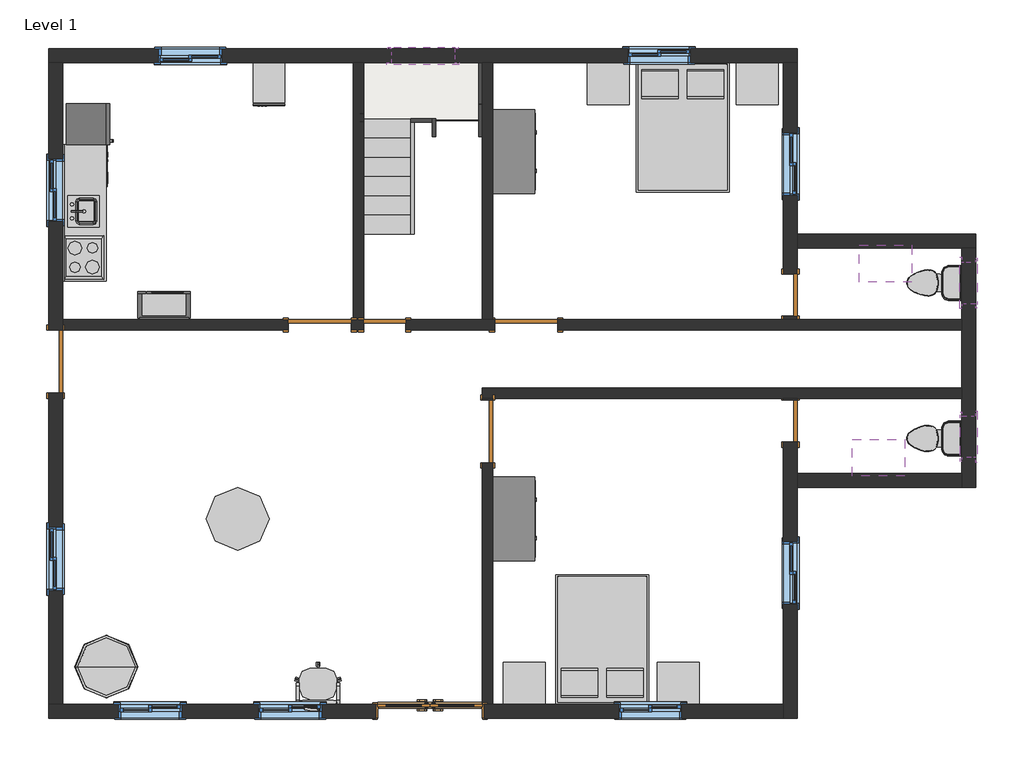
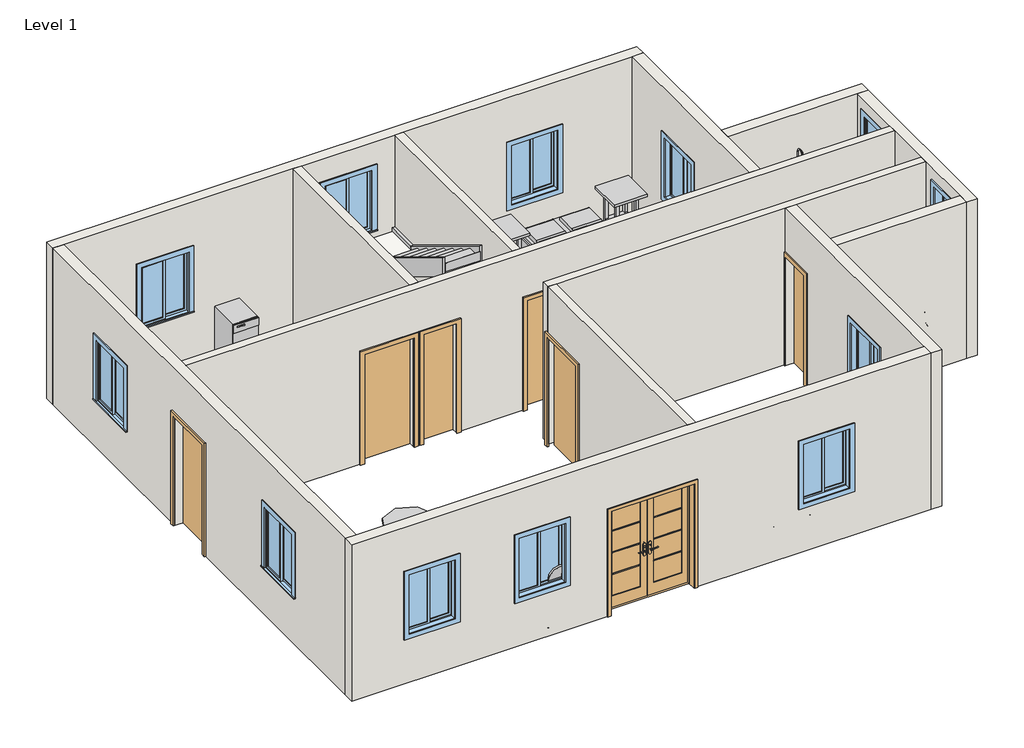
# One storey, incomplete: 13 walls, 12 furniture elements, 12 windows, 8 doors, 8 members, 6 proxies, 5 flow terminals, 2 stair flights, 1 slab.
"""IFC4 building model written with IfcOpenShell, lengths in millimetres."""

from ifc_helpers import new_model, si_unit, frame, origin, origin_with_axes, place, context, project, spatial, polyline, outline, extrude, faceted_brep, transform, mapped, element, save
from components import proxy_7e1014cc, proxy_a6faaae8, proxy_45b28599, kitchenette_medium_kitchenette_medium_844211aa, proxy_8a8d5ab2, proxy_c523a7b7, door_b03bd389, door_16372e1c, door_686f89d2, door_719f80de, single_flush_inner_door_2_1112daf7, single_flush_inner_door_2_89112ad5, single_flush_inner_door_2_5ca4d175, flow_terminal_871c2e40, flow_terminal_38af2918, toilet_domestic_3d_toilet_domestic_3d_f7549cf7, toilet_domestic_3d_toilet_domestic_3d_183bbd19, furniture_c8abb964, chair_executive_chair_executive_8d69e98c, furniture_c6510c7c, furniture_9fa109b2, furniture_905aceb5, furniture_5bc9ed15, furniture_c80d6d9c, non_monolithic_landing_d6ac0f27, stair_flight_b26bc1e7, stair_flight_d75c07b6, window_54100e87, window_e41d21a6

model = new_model("IFC4")

# Units and contexts
model_context = context("Model", 3, world=origin())
ifc_project = project(units=[si_unit("LENGTHUNIT", "METRE", prefix="MILLI")], contexts=[model_context])

# Site, building, storey
site = spatial("IfcSite", under=ifc_project)
building = spatial("IfcBuilding", under=site)
storey = spatial("IfcBuildingStorey", under=building, Name="Level 1", Elevation=0.0)

# Proxies
placement = place(None, origin())
proxy_shape = proxy_7e1014cc(model_context)
element("IfcBuildingElementProxy", 1, Name="18\" x 24\" x 34 1/2\"", ObjectType="18\" x 24\" x 34 1/2\"", at=placement, inside=storey, context=model_context, shape_type="MappedRepresentation", body=[
    mapped(proxy_shape, transform((-11897.4467487, 9092.6021187, 0.0), x_axis=(1.0, 0.0, 0.0), y_axis=(0.0, 1.0, 0.0), z_axis=(0.0, 0.0, 1.0))),
])
proxy_2_shape = proxy_a6faaae8(model_context)
element("IfcBuildingElementProxy", 2, Name="Cook Top-4 Unit2 : 22\" x 20\"", ObjectType="Cook Top-4 Unit2 : 22\" x 20\"", at=placement, inside=storey, context=model_context, shape_type="MappedRepresentation", body=[
    mapped(proxy_2_shape, transform((-14283.7292802, 6831.7516835, 0.0), x_axis=(0.0, 1.0000000000000002, 0.0), y_axis=(-1.0000000000000002, 0.0, 0.0), z_axis=(0.0, 0.0, 1.0))),
])
proxy_3_shape = proxy_45b28599(model_context)
element("IfcBuildingElementProxy", 3, Name="Dishwasher : 24\" x 24\" x 34\"", ObjectType="Dishwasher : 24\" x 24\" x 34\"", at=placement, inside=storey, context=model_context, shape_type="MappedRepresentation", body=[
    mapped(proxy_3_shape, transform((-13991.8797154, 7782.934215, 0.0), x_axis=(0.0, 1.0000000000000002, 0.0), y_axis=(-1.0000000000000002, 0.0, 0.0), z_axis=(0.0, 0.0, 1.0))),
])
kitchenette_medium_kitchenette_medium_shape = kitchenette_medium_kitchenette_medium_844211aa(model_context)
element("IfcBuildingElementProxy", 4, Name="Kitchenette - Medium : Kitchenette - Medium", ObjectType="Kitchenette - Medium : Kitchenette - Medium", at=placement, inside=storey, context=model_context, shape_type="MappedRepresentation", body=[
    mapped(kitchenette_medium_kitchenette_medium_shape, transform((-14588.5292802, 7155.9139786, 0.0), x_axis=(0.0, 1.0000000000000002, 0.0), y_axis=(-1.0000000000000002, 0.0, 0.0), z_axis=(0.0, 0.0, 1.0))),
])
proxy_4_shape = proxy_8a8d5ab2(model_context)
element("IfcBuildingElementProxy", 5, Name="Microwave : 30\" x 16\" x 18\"", ObjectType="Microwave : 30\" x 16\" x 18\"", at=placement, inside=storey, context=model_context, shape_type="MappedRepresentation", body=[
    mapped(proxy_4_shape, transform((-12615.0364029, 5780.1711777, 0.0), x_axis=(-1.0000000000000004, 0.0, 0.0), y_axis=(0.0, -1.0000000000000004, 0.0), z_axis=(0.0, 0.0, 1.0))),
])
proxy_5_shape = proxy_c523a7b7(model_context)
element("IfcBuildingElementProxy", 6, Name="Refrigerator : 24\" x 25\" LH", ObjectType="Refrigerator : 24\" x 25\" LH", at=placement, inside=storey, context=model_context, shape_type="MappedRepresentation", body=[
    mapped(proxy_5_shape, transform((-14238.0803087, 8768.5016835, 0.0), x_axis=(0.0, 1.0000000000000002, 0.0), y_axis=(-1.0000000000000002, 0.0, 0.0), z_axis=(0.0, 0.0, 1.0))),
])

# Doors
door_shape = door_b03bd389(model_context)
element("IfcDoor", 7, ObjectType="Door-Exterior-Double-Full Glass-Wood_Clad : 60\" x 80\"", at=placement, inside=storey, context=model_context, shape_type="MappedRepresentation", body=[
    mapped(door_shape, transform((-9254.5292802, 243.6266835, 0.0), x_axis=(1.0, 0.0, 0.0), y_axis=(0.0, 1.0, 0.0), z_axis=(0.0, 0.0, 1.0))),
])
door_2_shape = door_16372e1c(model_context)
element("IfcDoor", 8, ObjectType="Single-Flush : 36\" x 84\"", at=placement, inside=storey, context=model_context, shape_type="MappedRepresentation", body=[
    mapped(door_2_shape, transform((-10854.7292802, 5853.8516835, 0.0), x_axis=(1.0, 0.0, 0.0), y_axis=(0.0, 1.0, 0.0), z_axis=(0.0, 0.0, 1.0))),
])
door_3_shape = door_686f89d2(model_context)
element("IfcDoor", 9, ObjectType="Single-Flush : 36\" x 84\"", at=placement, inside=storey, context=model_context, shape_type="MappedRepresentation", body=[
    mapped(door_3_shape, transform((-7857.5292802, 5853.8516835, 0.0), x_axis=(-1.0, 0.0, 0.0), y_axis=(0.0, -1.0, 0.0), z_axis=(0.0, 0.0, 1.0))),
])
element("IfcDoor", 10, ObjectType="Single-Flush : 36\" x 84\"", at=placement, inside=storey, context=model_context, shape_type="MappedRepresentation", body=[
    mapped(door_3_shape, transform((-8416.3292802, 4304.4516835, -50.8), x_axis=(0.0, 1.0, 0.0), y_axis=(-1.0, 0.0, 0.0), z_axis=(0.0, 0.0, 1.0))),
])
door_4_shape = door_719f80de(model_context)
element("IfcDoor", 11, ObjectType="Single-Flush : 36\" x 84\"", at=placement, inside=storey, context=model_context, shape_type="MappedRepresentation", body=[
    mapped(door_4_shape, transform((-14690.1292802, 5320.4516835, 0.0), x_axis=(0.0, 1.0, 0.0), y_axis=(-1.0, 0.0, 0.0), z_axis=(0.0, 0.0, 1.0))),
])
single_flush_inner_door_2_shape = single_flush_inner_door_2_1112daf7(model_context)
element("IfcDoor", 12, ObjectType="Single-Flush : inner door 2", at=placement, inside=storey, context=model_context, shape_type="MappedRepresentation", body=[
    mapped(single_flush_inner_door_2_shape, transform((-4022.1292802, 4456.8516835, 0.0), x_axis=(0.0, 1.0, 0.0), y_axis=(-1.0, 0.0, 0.0), z_axis=(0.0, 0.0, 1.0))),
])
single_flush_inner_door_2_2_shape = single_flush_inner_door_2_89112ad5(model_context)
element("IfcDoor", 13, ObjectType="Single-Flush : inner door 2", at=placement, inside=storey, context=model_context, shape_type="MappedRepresentation", body=[
    mapped(single_flush_inner_door_2_2_shape, transform((-4022.1292802, 6285.6516835, 0.0), x_axis=(0.0, -1.0, 0.0), y_axis=(1.0, 0.0, 0.0), z_axis=(0.0, 0.0, 1.0))),
])
single_flush_inner_door_2_3_shape = single_flush_inner_door_2_5ca4d175(model_context)
element("IfcDoor", 14, ObjectType="Single-Flush : inner door 2", at=placement, inside=storey, context=model_context, shape_type="MappedRepresentation", body=[
    mapped(single_flush_inner_door_2_3_shape, transform((-9914.9292802, 5853.8516835, 0.0), x_axis=(-1.0, 0.0, 0.0), y_axis=(0.0, -1.0, 0.0), z_axis=(0.0, 0.0, 1.0))),
])

# Flow terminals
flow_terminal_shape = flow_terminal_871c2e40(model_context)
element("IfcFlowTerminal", 15, ObjectType="Sink Kitchen-Island : 18\" x 18\"", at=placement, inside=storey, context=model_context, shape_type="MappedRepresentation", body=[
    mapped(flow_terminal_shape, transform((-14281.3838791, 7489.162443, -14.4), x_axis=(0.0, 1.0000000000000002, 0.0), y_axis=(-1.0000000000000002, 0.0, 0.0), z_axis=(0.0, 0.0, 1.0))),
])
flow_terminal_2_shape = flow_terminal_38af2918(model_context)
element("IfcFlowTerminal", 16, ObjectType="Sink Kitchen-Single : 30\" x 21\"", at=placement, inside=storey, context=model_context, shape_type="MappedRepresentation", body=[
    mapped(flow_terminal_2_shape, transform((-2723.7400396, 3925.7970846, 1219.2), x_axis=(-1.0000000000000002, 0.0, 0.0), y_axis=(0.0, -1.0000000000000002, 0.0), z_axis=(0.0, 0.0, 1.0))),
])
element("IfcFlowTerminal", 17, ObjectType="Sink Kitchen-Single : 30\" x 21\"", at=placement, inside=storey, context=model_context, shape_type="MappedRepresentation", body=[
    mapped(flow_terminal_2_shape, transform((-2653.5185208, 6740.5062824, 1219.2), x_axis=(1.0, 0.0, 0.0), y_axis=(0.0, 1.0, 0.0), z_axis=(0.0, 0.0, 1.0))),
])
toilet_domestic_3d_toilet_domestic_3d_shape = toilet_domestic_3d_toilet_domestic_3d_f7549cf7(model_context)
toilet_domestic_3d_toilet_domestic_3d_2_shape = toilet_domestic_3d_toilet_domestic_3d_183bbd19(model_context)
element("IfcFlowTerminal", 18, ObjectType="Toilet-Domestic-3D : Toilet-Domestic-3D", at=placement, inside=storey, context=model_context, shape_type="MappedRepresentation", body=[
    mapped(toilet_domestic_3d_toilet_domestic_3d_shape, transform((-2027.6253076, 4202.8516835, 0.0), x_axis=(0.0, -1.0, 0.0), y_axis=(1.0, 0.0, 0.0), z_axis=(0.0, 0.0, 1.0))),
    mapped(toilet_domestic_3d_toilet_domestic_3d_2_shape, transform((-2027.6253076, 4202.8516835, 0.0), x_axis=(0.0, -1.0, 0.0), y_axis=(1.0, 0.0, 0.0), z_axis=(0.0, 0.0, 1.0))),
])
element("IfcFlowTerminal", 19, ObjectType="Toilet-Domestic-3D : Toilet-Domestic-3D", at=placement, inside=storey, context=model_context, shape_type="MappedRepresentation", body=[
    mapped(toilet_domestic_3d_toilet_domestic_3d_shape, transform((-2027.6253076, 6463.4516835, 0.0), x_axis=(0.0, -1.0, 0.0), y_axis=(1.0, 0.0, 0.0), z_axis=(0.0, 0.0, 1.0))),
    mapped(toilet_domestic_3d_toilet_domestic_3d_2_shape, transform((-2027.6253076, 6463.4516835, 0.0), x_axis=(0.0, -1.0, 0.0), y_axis=(1.0, 0.0, 0.0), z_axis=(0.0, 0.0, 1.0))),
])

# Furniture
furniture_shape = furniture_c8abb964(model_context)
element("IfcFurniture", 20, ObjectType="Bed-Box : Double 53\" x 74\"", at=placement, inside=storey, context=model_context, shape_type="MappedRepresentation", body=[
    mapped(furniture_shape, transform((-5923.3817392, 8958.4811917, 0.0), x_axis=(1.0, 0.0, 0.0), y_axis=(0.0, 1.0, 0.0), z_axis=(0.0, 0.0, 1.0))),
])
element("IfcFurniture", 21, ObjectType="Bed-Box : Double 53\" x 74\"", at=placement, inside=storey, context=model_context, shape_type="MappedRepresentation", body=[
    mapped(furniture_shape, transform((-6413.4768212, 1047.4221753, 0.0), x_axis=(-0.9999999999999998, 0.0, 0.0), y_axis=(0.0, -0.9999999999999998, 0.0), z_axis=(0.0, 0.0, 1.0))),
])
chair_executive_chair_executive_shape = chair_executive_chair_executive_8d69e98c(model_context)
element("IfcFurniture", 22, ObjectType="Chair-Executive : Chair-Executive", at=placement, inside=storey, context=model_context, shape_type="MappedRepresentation", body=[
    mapped(chair_executive_chair_executive_shape, transform((-11021.1200999, 583.4557819, 0.0), x_axis=(1.0000000000000007, 0.0, 0.0), y_axis=(0.0, 1.0000000000000007, 0.0), z_axis=(0.0, 0.0, 1.0))),
])
furniture_2_shape = furniture_c6510c7c(model_context)
element("IfcFurniture", 23, ObjectType="Counter Top w Sink Hole : 24\" Depth", at=placement, inside=storey, context=model_context, shape_type="MappedRepresentation", body=[
    mapped(furniture_2_shape, transform((-14588.5292802, 7689.3139786, -14.4), x_axis=(0.0, 1.0000000000000002, 0.0), y_axis=(-1.0000000000000002, 0.0, 0.0), z_axis=(0.0, 0.0, 1.0))),
])
furniture_3_shape = furniture_9fa109b2(model_context)
element("IfcFurniture", 24, ObjectType="Dresser : 48\" x 72\" x 24\"", at=placement, inside=storey, context=model_context, shape_type="MappedRepresentation", body=[
    mapped(furniture_3_shape, transform((-8398.4922343, 3303.6449434, 0.0), x_axis=(0.0, 1.0000000000000009, 0.0), y_axis=(-1.0000000000000009, 0.0, 0.0), z_axis=(0.0, 0.0, 1.0))),
])
element("IfcFurniture", 25, ObjectType="Dresser : 48\" x 72\" x 24\"", at=placement, inside=storey, context=model_context, shape_type="MappedRepresentation", body=[
    mapped(furniture_3_shape, transform((-8398.4922343, 8637.6449434, 0.0), x_axis=(0.0, 1.0000000000000002, 0.0), y_axis=(-1.0000000000000002, 0.0, 0.0), z_axis=(0.0, 0.0, 1.0))),
])
furniture_4_shape = furniture_905aceb5(model_context)
element("IfcFurniture", 26, ObjectType="Table-Dining Round w Chairs : 36\" Diameter", at=placement, inside=storey, context=model_context, shape_type="MappedRepresentation", body=[
    mapped(furniture_4_shape, transform((-12152.2112474, 3219.3303721, 0.0), x_axis=(1.0, 0.0, 0.0), y_axis=(0.0, 1.0, 0.0), z_axis=(0.0, 0.0, 1.0))),
])
furniture_5_shape = furniture_5bc9ed15(model_context)
element("IfcFurniture", 27, ObjectType="Table-Night Stand : 24\" x 24\" x 30\"", at=placement, inside=storey, context=model_context, shape_type="MappedRepresentation", body=[
    mapped(furniture_5_shape, transform((-8191.4629105, 342.0516835, 0.0), x_axis=(1.0, 0.0, 0.0), y_axis=(0.0, 1.0, 0.0), z_axis=(0.0, 0.0, 1.0))),
])
element("IfcFurniture", 28, ObjectType="Table-Night Stand : 24\" x 24\" x 30\"", at=placement, inside=storey, context=model_context, shape_type="MappedRepresentation", body=[
    mapped(furniture_5_shape, transform((-5956.2629105, 342.0516835, 0.0), x_axis=(1.0, 0.0, 0.0), y_axis=(0.0, 1.0, 0.0), z_axis=(0.0, 0.0, 1.0))),
])
element("IfcFurniture", 29, ObjectType="Table-Night Stand : 24\" x 24\" x 30\"", at=placement, inside=storey, context=model_context, shape_type="MappedRepresentation", body=[
    mapped(furniture_5_shape, transform((-4813.2629105, 9054.2516835, 0.0), x_axis=(1.0, 0.0, 0.0), y_axis=(0.0, 1.0, 0.0), z_axis=(0.0, 0.0, 1.0))),
])
element("IfcFurniture", 30, ObjectType="Table-Night Stand : 24\" x 24\" x 30\"", at=placement, inside=storey, context=model_context, shape_type="MappedRepresentation", body=[
    mapped(furniture_5_shape, transform((-6972.2629105, 9054.2516835, 0.0), x_axis=(1.0, 0.0, 0.0), y_axis=(0.0, 1.0, 0.0), z_axis=(0.0, 0.0, 1.0))),
])
furniture_6_shape = furniture_c80d6d9c(model_context)
element("IfcFurniture", 31, ObjectType="Table-Round : 36\" Diameter", at=placement, inside=storey, context=model_context, shape_type="MappedRepresentation", body=[
    mapped(furniture_6_shape, transform((-13953.5292802, 888.1516835, 0.0), x_axis=(1.0, 0.0, 0.0), y_axis=(0.0, 1.0, 0.0), z_axis=(0.0, 0.0, 1.0))),
])

# Members
element("IfcMember", 32, ObjectType="Stringer - 2\" Width", at=placement, inside=storey, context=model_context, shape_type="SweptSolid", body=[
    extrude(outline(polyline([(7174.6516835, 0.0), (7174.6516835, 212.114512), (8906.1927388, 1261.5333333), (8991.3471953, 956.7333333), (7412.7371953, 0.0), (7174.6516835, 0.0)])), frame((-10270.5292802, 0.0, 0.0), z_axis=(1.0, 0.0, 0.0), x_axis=(0.0, 1.0, 0.0)), (0.0, 0.0, 1.0), 50.8),
])
element("IfcMember", 33, ObjectType="Stringer - 2\" Width", at=placement, inside=storey, context=model_context, shape_type="SweptSolid", body=[
    extrude(outline(polyline([(7174.6516835, 0.0), (7174.6516835, 212.114512), (8800.2516835, 1197.3266332), (8800.2516835, 840.9178717), (7412.7371953, 0.0), (7174.6516835, 0.0)])), frame((-9533.9292802, 0.0, 0.0), z_axis=(1.0, 0.0, 0.0), x_axis=(0.0, 1.0, 0.0)), (0.0, 0.0, 1.0), 50.8),
])
element("IfcMember", 34, ObjectType="Stringer - 2\" Width", at=placement, inside=storey, context=model_context, shape_type="SweptSolid", body=[
    extrude(outline(polyline([(9075.3106283, 1261.5333333), (8990.1561718, 956.7333333), (6895.2516835, 2226.3724171), (6895.2516835, 2582.7811786), (9075.3106283, 1261.5333333)])), frame((-8543.3292802, 0.0, 0.0), z_axis=(1.0, 0.0, 0.0), x_axis=(0.0, 1.0, 0.0)), (0.0, 0.0, 1.0), 50.8),
])
element("IfcMember", 35, ObjectType="Stringer - 2\" Width", at=placement, inside=storey, context=model_context, shape_type="SweptSolid", body=[
    extrude(outline(polyline([(8851.0516835, 1397.4478453), (8851.0516835, 1041.0390838), (6895.2516835, 2226.3724171), (6895.2516835, 2582.7811786), (8851.0516835, 1397.4478453)])), frame((-9220.7689718, 0.0, 0.0), z_axis=(1.0, 0.0, 0.0), x_axis=(0.0, 1.0, 0.0)), (0.0, 0.0, 1.0), 50.8),
])
element("IfcMember", 36, ObjectType="Stringer - 2\" Width", at=placement, inside=storey, context=model_context, shape_type="Brep", body=[
    faceted_brep([(-8543.3292802, 9075.3106283, 1261.5333333), (-8492.5292802, 9075.3106283, 1261.5333333), (-8492.5292802, 9816.2516835, 1261.5333333), (-8543.3292802, 9765.4516835, 1261.5333333), (-8543.3292802, 8990.1561718, 956.7333333), (-8543.3292802, 9765.4516835, 956.7333333), (-8492.5292802, 8990.1561718, 956.7333333), (-8492.5292802, 9816.2516835, 956.7333333)], [[[0, 1, 2, 3]], [[4, 0, 3, 5]], [[6, 4, 5, 7]], [[1, 6, 7, 2]], [[1, 0, 4, 6]], [[2, 7, 5, 3]]]),
])
element("IfcMember", 37, ObjectType="Stringer - 2\" Width", at=placement, inside=storey, context=model_context, shape_type="SweptSolid", body=[
    extrude(outline(polyline([(-8492.5292802, 9816.2516835), (-8543.3292802, 9765.4516835), (-10219.7292802, 9765.4516835), (-10270.5292802, 9816.2516835), (-8492.5292802, 9816.2516835)])), frame((0.0, 0.0, 956.7333333), z_axis=(0.0, 0.0, 1.0), x_axis=(1.0, 0.0, 0.0)), (0.0, 0.0, 1.0), 304.8),
])
element("IfcMember", 38, ObjectType="Stringer - 2\" Width", at=placement, inside=storey, context=model_context, shape_type="Brep", body=[
    faceted_brep([(-10219.7292802, 9765.4516835, 1261.5333333), (-10270.5292802, 9816.2516835, 1261.5333333), (-10270.5292802, 8906.1927388, 1261.5333333), (-10219.7292802, 8906.1927388, 1261.5333333), (-10219.7292802, 9765.4516835, 956.7333333), (-10219.7292802, 8991.3471953, 956.7333333), (-10270.5292802, 9816.2516835, 956.7333333), (-10270.5292802, 8991.3471953, 956.7333333)], [[[0, 1, 2, 3]], [[4, 0, 3, 5]], [[6, 4, 5, 7]], [[1, 6, 7, 2]], [[1, 0, 4, 6]], [[2, 7, 5, 3]]]),
])
element("IfcMember", 39, ObjectType="Stringer - 2\" Width", at=placement, inside=storey, context=model_context, shape_type="SweptSolid", body=[
    extrude(outline(polyline([(-9533.9292802, 8800.2516835), (-9533.9292802, 8851.0516835), (-9220.7689718, 8851.0516835), (-9220.7689718, 8800.2516835), (-9533.9292802, 8800.2516835)])), frame((0.0, 0.0, 956.7333333), z_axis=(0.0, 0.0, 1.0), x_axis=(1.0, 0.0, 0.0)), (0.0, 0.0, 1.0), 304.8),
])

# Slab
non_monolithic_landing_shape = non_monolithic_landing_d6ac0f27(model_context)
element("IfcSlab", 40, ObjectType="Non-Monolithic Landing", at=placement, inside=storey, context=model_context, shape_type="MappedRepresentation", body=[
    mapped(non_monolithic_landing_shape, transform((0.0, 0.0, 0.0), x_axis=(1.0, 0.0, 0.0), y_axis=(0.0, 1.0, 0.0), z_axis=(0.0, 0.0, 1.0))),
])

# Stair flights
stair_flight_shape = stair_flight_b26bc1e7(model_context)
element("IfcStairFlight", 41, ObjectType="2\" Tread 1\" Nosing 1/4\" Riser", at=placement, inside=storey, context=model_context, shape_type="MappedRepresentation", body=[
    mapped(stair_flight_shape, transform((0.0, 0.0, 0.0), x_axis=(1.0, 0.0, 0.0), y_axis=(0.0, 1.0, 0.0), z_axis=(0.0, 0.0, 1.0))),
])
stair_flight_2_shape = stair_flight_d75c07b6(model_context)
element("IfcStairFlight", 42, ObjectType="2\" Tread 1\" Nosing 1/4\" Riser", at=placement, inside=storey, context=model_context, shape_type="MappedRepresentation", body=[
    mapped(stair_flight_2_shape, transform((0.0, 0.0, 0.0), x_axis=(1.0, 0.0, 0.0), y_axis=(0.0, 1.0, 0.0), z_axis=(0.0, 0.0, 1.0))),
])

# Walls
element("IfcWall", 43, ObjectType="Generic - 8\"", at=placement, inside=storey, context=model_context, shape_type="Brep", body=[
    faceted_brep([(-14791.7292802, 9663.8516835, 0.0), (-14588.5292802, 9663.8516835, 0.0), (-10372.1292802, 9663.8516835, 0.0), (-10219.7292802, 9663.8516835, 0.0), (-8492.5292802, 9663.8516835, 0.0), (-8340.1292802, 9663.8516835, 0.0), (-4123.7292802, 9663.8516835, 0.0), (-3920.5292802, 9663.8516835, 0.0), (-3920.5292802, 9663.8516835, 3048.0), (-4123.7292802, 9663.8516835, 3048.0), (-8340.1292802, 9663.8516835, 3048.0), (-8492.5292802, 9663.8516835, 3048.0), (-10219.7292802, 9663.8516835, 3048.0), (-10372.1292802, 9663.8516835, 3048.0), (-14588.5292802, 9663.8516835, 3048.0), (-14791.7292802, 9663.8516835, 3048.0), (-13191.5292802, 9663.8516835, 2133.6), (-12277.1292802, 9663.8516835, 2133.6), (-12277.1292802, 9663.8516835, 914.4), (-13191.5292802, 9663.8516835, 914.4), (-9813.3292802, 9663.8516835, 2540.0), (-8898.9292802, 9663.8516835, 2540.0), (-8898.9292802, 9663.8516835, 1320.8), (-9813.3292802, 9663.8516835, 1320.8), (-5469.9292802, 9663.8516835, 2133.6), (-5469.9292802, 9663.8516835, 914.4), (-6384.3292802, 9663.8516835, 914.4), (-6384.3292802, 9663.8516835, 2133.6), (-14791.7292802, 9867.0516835, 0.0), (-14791.7292802, 9867.0516835, 3048.0), (-3920.5292802, 9867.0516835, 3048.0), (-3920.5292802, 9867.0516835, 0.0), (-13191.5292802, 9867.0516835, 2133.6), (-13191.5292802, 9867.0516835, 914.4), (-12277.1292802, 9867.0516835, 914.4), (-12277.1292802, 9867.0516835, 2133.6), (-9813.3292802, 9867.0516835, 2540.0), (-9813.3292802, 9867.0516835, 1320.8), (-8898.9292802, 9867.0516835, 1320.8), (-8898.9292802, 9867.0516835, 2540.0), (-5469.9292802, 9867.0516835, 2133.6), (-6384.3292802, 9867.0516835, 2133.6), (-6384.3292802, 9867.0516835, 914.4), (-5469.9292802, 9867.0516835, 914.4)], [[[0, 1, 2, 3, 4, 5, 6, 7, 8, 9, 10, 11, 12, 13, 14, 15], [16, 17, 18, 19], [20, 21, 22, 23], [24, 25, 26, 27]], [[28, 29, 30, 31], [32, 33, 34, 35], [36, 37, 38, 39], [40, 41, 42, 43]], [[7, 6, 5, 4, 3, 2, 1, 0, 28, 31]], [[15, 14, 13, 12, 11, 10, 9, 8, 30, 29]], [[8, 7, 31, 30]], [[0, 15, 29, 28]], [[33, 32, 16, 19]], [[34, 33, 19, 18]], [[35, 34, 18, 17]], [[32, 35, 17, 16]], [[37, 36, 20, 23]], [[38, 37, 23, 22]], [[39, 38, 22, 21]], [[36, 39, 21, 20]], [[25, 24, 40, 43]], [[26, 25, 43, 42]], [[27, 26, 42, 41]], [[24, 27, 41, 40]]]),
])
element("IfcWall", 44, ObjectType="Generic - 8\"", at=placement, inside=storey, context=model_context, shape_type="Brep", body=[
    faceted_brep([(-4123.7292802, 5930.0516835, 3048.0), (-4123.7292802, 9663.8516835, 3048.0), (-4123.7292802, 9663.8516835, 0.0), (-4123.7292802, 6590.4516835, 0.0), (-4123.7292802, 6590.4516835, 2133.6), (-4123.7292802, 5980.8516835, 2133.6), (-4123.7292802, 5980.8516835, 0.0), (-4123.7292802, 5930.0516835, 0.0), (-4123.7292802, 7733.4516835, 2133.6), (-4123.7292802, 7733.4516835, 914.4), (-4123.7292802, 8647.8516835, 914.4), (-4123.7292802, 8647.8516835, 2133.6), (-3920.5292802, 9663.8516835, 3048.0), (-3920.5292802, 7174.6516835, 3048.0), (-3920.5292802, 6971.4516835, 3048.0), (-3920.5292802, 5930.0516835, 3048.0), (-3920.5292802, 5930.0516835, 0.0), (-3920.5292802, 5980.8516835, 0.0), (-3920.5292802, 5980.8516835, 2133.6), (-3920.5292802, 6590.4516835, 2133.6), (-3920.5292802, 6590.4516835, 0.0), (-3920.5292802, 6971.4516835, 0.0), (-3920.5292802, 7174.6516835, 0.0), (-3920.5292802, 9663.8516835, 0.0), (-3920.5292802, 7733.4516835, 2133.6), (-3920.5292802, 8647.8516835, 2133.6), (-3920.5292802, 8647.8516835, 914.4), (-3920.5292802, 7733.4516835, 914.4)], [[[0, 1, 2, 3, 4, 5, 6, 7], [8, 9, 10, 11]], [[12, 13, 14, 15, 16, 17, 18, 19, 20, 21, 22, 23], [24, 25, 26, 27]], [[2, 23, 22, 21, 20, 3]], [[16, 7, 6, 17]], [[1, 0, 15, 14, 13, 12]], [[2, 1, 12, 23]], [[0, 7, 16, 15]], [[18, 5, 4, 19]], [[19, 4, 3, 20]], [[9, 8, 24, 27]], [[10, 9, 27, 26]], [[11, 10, 26, 25]], [[8, 11, 25, 24]], [[5, 18, 17, 6]]]),
])
element("IfcWall", 45, ObjectType="Generic - 8\"", at=placement, inside=storey, context=model_context, shape_type="Brep", body=[
    faceted_brep([(-14791.7292802, 342.0516835, 3048.0), (-14588.5292802, 342.0516835, 3048.0), (-8492.5292802, 342.0516835, 3048.0), (-8340.1292802, 342.0516835, 3048.0), (-4123.7292802, 342.0516835, 3048.0), (-4123.7292802, 342.0516835, 0.0), (-8340.1292802, 342.0516835, 0.0), (-8467.1292802, 342.0516835, 0.0), (-8467.1292802, 342.0516835, 2057.4), (-10041.9292802, 342.0516835, 2057.4), (-10041.9292802, 342.0516835, 0.0), (-14588.5292802, 342.0516835, 0.0), (-14791.7292802, 342.0516835, 0.0), (-10829.3292802, 342.0516835, 2133.6), (-11743.7292802, 342.0516835, 2133.6), (-11743.7292802, 342.0516835, 914.4), (-10829.3292802, 342.0516835, 914.4), (-12861.3292802, 342.0516835, 2133.6), (-13775.7292802, 342.0516835, 2133.6), (-13775.7292802, 342.0516835, 914.4), (-12861.3292802, 342.0516835, 914.4), (-5596.9292802, 342.0516835, 2133.6), (-6511.3292802, 342.0516835, 2133.6), (-6511.3292802, 342.0516835, 914.4), (-5596.9292802, 342.0516835, 914.4), (-4123.7292802, 138.8516835, 3048.0), (-14791.7292802, 138.8516835, 3048.0), (-14791.7292802, 138.8516835, 0.0), (-10041.9292802, 138.8516835, 0.0), (-10041.9292802, 138.8516835, 2057.4), (-8467.1292802, 138.8516835, 2057.4), (-8467.1292802, 138.8516835, 0.0), (-4123.7292802, 138.8516835, 0.0), (-10829.3292802, 138.8516835, 2133.6), (-10829.3292802, 138.8516835, 914.4), (-11743.7292802, 138.8516835, 914.4), (-11743.7292802, 138.8516835, 2133.6), (-12861.3292802, 138.8516835, 2133.6), (-12861.3292802, 138.8516835, 914.4), (-13775.7292802, 138.8516835, 914.4), (-13775.7292802, 138.8516835, 2133.6), (-5596.9292802, 138.8516835, 2133.6), (-5596.9292802, 138.8516835, 914.4), (-6511.3292802, 138.8516835, 914.4), (-6511.3292802, 138.8516835, 2133.6)], [[[0, 1, 2, 3, 4, 5, 6, 7, 8, 9, 10, 11, 12], [13, 14, 15, 16], [17, 18, 19, 20], [21, 22, 23, 24]], [[25, 26, 27, 28, 29, 30, 31, 32], [33, 34, 35, 36], [37, 38, 39, 40], [41, 42, 43, 44]], [[5, 32, 31, 7, 6]], [[27, 12, 11, 10, 28]], [[4, 3, 2, 1, 0, 26, 25]], [[5, 4, 25, 32]], [[0, 12, 27, 26]], [[30, 8, 7, 31]], [[8, 30, 29, 9]], [[9, 29, 28, 10]], [[34, 33, 13, 16]], [[35, 34, 16, 15]], [[36, 35, 15, 14]], [[33, 36, 14, 13]], [[38, 37, 17, 20]], [[39, 38, 20, 19]], [[40, 39, 19, 18]], [[37, 40, 18, 17]], [[42, 41, 21, 24]], [[43, 42, 24, 23]], [[44, 43, 23, 22]], [[41, 44, 22, 21]]]),
])
element("IfcWall", 46, ObjectType="Generic - 8\"", at=placement, inside=storey, context=model_context, shape_type="Brep", body=[
    faceted_brep([(-14588.5292802, 5777.6516835, 2133.6), (-14588.5292802, 5777.6516835, 0.0), (-14588.5292802, 5930.0516835, 0.0), (-14588.5292802, 9663.8516835, 0.0), (-14588.5292802, 9663.8516835, 3048.0), (-14588.5292802, 5930.0516835, 3048.0), (-14588.5292802, 5777.6516835, 3048.0), (-14588.5292802, 342.0516835, 3048.0), (-14588.5292802, 342.0516835, 0.0), (-14588.5292802, 4863.2516835, 0.0), (-14588.5292802, 4863.2516835, 2133.6), (-14588.5292802, 2907.4516835, 2133.6), (-14588.5292802, 2907.4516835, 914.4), (-14588.5292802, 1993.0516835, 914.4), (-14588.5292802, 1993.0516835, 2133.6), (-14588.5292802, 8266.8516835, 2133.6), (-14588.5292802, 8266.8516835, 914.4), (-14588.5292802, 7352.4516835, 914.4), (-14588.5292802, 7352.4516835, 2133.6), (-14791.7292802, 9663.8516835, 0.0), (-14791.7292802, 5777.6516835, 0.0), (-14791.7292802, 5777.6516835, 2133.6), (-14791.7292802, 4863.2516835, 2133.6), (-14791.7292802, 4863.2516835, 0.0), (-14791.7292802, 342.0516835, 0.0), (-14791.7292802, 342.0516835, 3048.0), (-14791.7292802, 9663.8516835, 3048.0), (-14791.7292802, 2907.4516835, 2133.6), (-14791.7292802, 1993.0516835, 2133.6), (-14791.7292802, 1993.0516835, 914.4), (-14791.7292802, 2907.4516835, 914.4), (-14791.7292802, 8266.8516835, 2133.6), (-14791.7292802, 7352.4516835, 2133.6), (-14791.7292802, 7352.4516835, 914.4), (-14791.7292802, 8266.8516835, 914.4)], [[[0, 1, 2, 3, 4, 5, 6, 7, 8, 9, 10], [11, 12, 13, 14], [15, 16, 17, 18]], [[19, 20, 21, 22, 23, 24, 25, 26], [27, 28, 29, 30], [31, 32, 33, 34]], [[9, 8, 24, 23]], [[3, 2, 1, 20, 19]], [[7, 6, 5, 4, 26, 25]], [[4, 3, 19, 26]], [[8, 7, 25, 24]], [[21, 20, 1, 0]], [[22, 21, 0, 10]], [[23, 22, 10, 9]], [[12, 11, 27, 30]], [[13, 12, 30, 29]], [[14, 13, 29, 28]], [[11, 14, 28, 27]], [[16, 15, 31, 34]], [[17, 16, 34, 33]], [[18, 17, 33, 32]], [[15, 18, 32, 31]]]),
])
element("IfcWall", 47, ObjectType="Generic - 8\"", at=placement, inside=storey, context=model_context, shape_type="Brep", body=[
    faceted_brep([(-3920.5292802, 6971.4516835, 0.0), (-1532.9292802, 6971.4516835, 0.0), (-1329.7292802, 6971.4516835, 0.0), (-1329.7292802, 6971.4516835, 3048.0), (-1532.9292802, 6971.4516835, 3048.0), (-3920.5292802, 6971.4516835, 3048.0), (-3920.5292802, 7174.6516835, 0.0), (-3920.5292802, 7174.6516835, 3048.0), (-1329.7292802, 7174.6516835, 3048.0), (-1329.7292802, 7174.6516835, 0.0)], [[[0, 1, 2, 3, 4, 5]], [[6, 7, 8, 9]], [[2, 1, 0, 6, 9]], [[5, 4, 3, 8, 7]], [[0, 5, 7, 6]], [[3, 2, 9, 8]]]),
])
element("IfcWall", 48, ObjectType="Generic - 8\"", at=placement, inside=storey, context=model_context, shape_type="Brep", body=[
    faceted_brep([(-1532.9292802, 6971.4516835, 0.0), (-1532.9292802, 5930.0516835, 0.0), (-1532.9292802, 5777.6516835, 0.0), (-1532.9292802, 4939.4516835, 0.0), (-1532.9292802, 4787.0516835, 0.0), (-1532.9292802, 3694.8516835, 0.0), (-1532.9292802, 3491.6516835, 0.0), (-1532.9292802, 3491.6516835, 3048.0), (-1532.9292802, 3694.8516835, 3048.0), (-1532.9292802, 4787.0516835, 3048.0), (-1532.9292802, 4939.4516835, 3048.0), (-1532.9292802, 5777.6516835, 3048.0), (-1532.9292802, 5930.0516835, 3048.0), (-1532.9292802, 6971.4516835, 3048.0), (-1532.9292802, 3923.4516835, 2768.6), (-1532.9292802, 3923.4516835, 2159.0), (-1532.9292802, 4533.0516835, 2159.0), (-1532.9292802, 4533.0516835, 2768.6), (-1532.9292802, 6768.2516835, 2768.6), (-1532.9292802, 6158.6516835, 2768.6), (-1532.9292802, 6158.6516835, 2159.0), (-1532.9292802, 6768.2516835, 2159.0), (-1329.7292802, 6971.4516835, 0.0), (-1329.7292802, 6971.4516835, 3048.0), (-1329.7292802, 3491.6516835, 3048.0), (-1329.7292802, 3491.6516835, 0.0), (-1329.7292802, 3923.4516835, 2768.6), (-1329.7292802, 4533.0516835, 2768.6), (-1329.7292802, 4533.0516835, 2159.0), (-1329.7292802, 3923.4516835, 2159.0), (-1329.7292802, 6768.2516835, 2768.6), (-1329.7292802, 6768.2516835, 2159.0), (-1329.7292802, 6158.6516835, 2159.0), (-1329.7292802, 6158.6516835, 2768.6)], [[[0, 1, 2, 3, 4, 5, 6, 7, 8, 9, 10, 11, 12, 13], [14, 15, 16, 17], [18, 19, 20, 21]], [[22, 23, 24, 25], [26, 27, 28, 29], [30, 31, 32, 33]], [[6, 5, 4, 3, 2, 1, 0, 22, 25]], [[13, 12, 11, 10, 9, 8, 7, 24, 23]], [[0, 13, 23, 22]], [[7, 6, 25, 24]], [[15, 14, 26, 29]], [[16, 15, 29, 28]], [[17, 16, 28, 27]], [[14, 17, 27, 26]], [[31, 30, 18, 21]], [[32, 31, 21, 20]], [[33, 32, 20, 19]], [[30, 33, 19, 18]]]),
])
element("IfcWall", 49, ObjectType="Generic - 8\"", at=placement, inside=storey, context=model_context, shape_type="SweptSolid", body=[
    extrude(outline(polyline([(-3920.5292802, 3694.8516835), (-1532.9292802, 3694.8516835), (-1532.9292802, 3491.6516835), (-3920.5292802, 3491.6516835), (-3920.5292802, 3694.8516835)])), origin_with_axes(), (0.0, 0.0, 1.0), 3048.0),
])
element("IfcWall", 50, ObjectType="Generic - 8\"", at=placement, inside=storey, context=model_context, shape_type="Brep", body=[
    faceted_brep([(-4123.7292802, 4787.0516835, 0.0), (-4123.7292802, 4761.6516835, 0.0), (-4123.7292802, 4761.6516835, 2133.6), (-4123.7292802, 4152.0516835, 2133.6), (-4123.7292802, 4152.0516835, 0.0), (-4123.7292802, 342.0516835, 0.0), (-4123.7292802, 138.8516835, 0.0), (-4123.7292802, 138.8516835, 3048.0), (-4123.7292802, 342.0516835, 3048.0), (-4123.7292802, 4787.0516835, 3048.0), (-4123.7292802, 1789.8516835, 2133.6), (-4123.7292802, 1789.8516835, 914.4), (-4123.7292802, 2704.2516835, 914.4), (-4123.7292802, 2704.2516835, 2133.6), (-3920.5292802, 4761.6516835, 2133.6), (-3920.5292802, 4761.6516835, 0.0), (-3920.5292802, 4787.0516835, 0.0), (-3920.5292802, 4787.0516835, 3048.0), (-3920.5292802, 3694.8516835, 3048.0), (-3920.5292802, 3491.6516835, 3048.0), (-3920.5292802, 138.8516835, 3048.0), (-3920.5292802, 138.8516835, 0.0), (-3920.5292802, 3491.6516835, 0.0), (-3920.5292802, 3694.8516835, 0.0), (-3920.5292802, 4152.0516835, 0.0), (-3920.5292802, 4152.0516835, 2133.6), (-3920.5292802, 1789.8516835, 2133.6), (-3920.5292802, 2704.2516835, 2133.6), (-3920.5292802, 2704.2516835, 914.4), (-3920.5292802, 1789.8516835, 914.4)], [[[0, 1, 2, 3, 4, 5, 6, 7, 8, 9], [10, 11, 12, 13]], [[14, 15, 16, 17, 18, 19, 20, 21, 22, 23, 24, 25], [26, 27, 28, 29]], [[16, 15, 1, 0]], [[24, 23, 22, 21, 6, 5, 4]], [[9, 8, 7, 20, 19, 18, 17]], [[7, 6, 21, 20]], [[0, 9, 17, 16]], [[2, 1, 15, 14]], [[3, 2, 14, 25]], [[4, 3, 25, 24]], [[11, 10, 26, 29]], [[12, 11, 29, 28]], [[13, 12, 28, 27]], [[10, 13, 27, 26]]]),
])
element("IfcWall", 51, ObjectType="inner wall", at=placement, inside=storey, context=model_context, shape_type="Brep", body=[
    faceted_brep([(-1532.9292802, 4939.4516835, 0.0), (-8492.5292802, 4939.4516835, 0.0), (-8492.5292802, 4939.4516835, 3048.0), (-1532.9292802, 4939.4516835, 3048.0), (-1532.9292802, 4787.0516835, 0.0), (-1532.9292802, 4787.0516835, 3048.0), (-3920.5292802, 4787.0516835, 3048.0), (-4123.7292802, 4787.0516835, 3048.0), (-8340.1292802, 4787.0516835, 3048.0), (-8492.5292802, 4787.0516835, 3048.0), (-8492.5292802, 4787.0516835, 0.0), (-8340.1292802, 4787.0516835, 0.0), (-4123.7292802, 4787.0516835, 0.0), (-3920.5292802, 4787.0516835, 0.0)], [[[0, 1, 2, 3]], [[4, 5, 6, 7, 8, 9, 10, 11, 12, 13]], [[1, 0, 4, 13, 12, 11, 10]], [[3, 2, 9, 8, 7, 6, 5]], [[0, 3, 5, 4]], [[2, 1, 10, 9]]]),
])
element("IfcWall", 52, ObjectType="inner wall", at=placement, inside=storey, context=model_context, shape_type="Brep", body=[
    faceted_brep([(-10219.7292802, 5930.0516835, 2133.6), (-10219.7292802, 5930.0516835, 0.0), (-10372.1292802, 5930.0516835, 0.0), (-10397.5292802, 5930.0516835, 0.0), (-10397.5292802, 5930.0516835, 2133.6), (-11311.9292802, 5930.0516835, 2133.6), (-11311.9292802, 5930.0516835, 0.0), (-14588.5292802, 5930.0516835, 0.0), (-14588.5292802, 5930.0516835, 3048.0), (-10372.1292802, 5930.0516835, 3048.0), (-10219.7292802, 5930.0516835, 3048.0), (-8492.5292802, 5930.0516835, 3048.0), (-8340.1292802, 5930.0516835, 3048.0), (-4123.7292802, 5930.0516835, 3048.0), (-3920.5292802, 5930.0516835, 3048.0), (-1532.9292802, 5930.0516835, 3048.0), (-1532.9292802, 5930.0516835, 0.0), (-3920.5292802, 5930.0516835, 0.0), (-4123.7292802, 5930.0516835, 0.0), (-7400.3292802, 5930.0516835, 0.0), (-7400.3292802, 5930.0516835, 2133.6), (-8314.7292802, 5930.0516835, 2133.6), (-8314.7292802, 5930.0516835, 0.0), (-8340.1292802, 5930.0516835, 0.0), (-8492.5292802, 5930.0516835, 0.0), (-9610.1292802, 5930.0516835, 0.0), (-9610.1292802, 5930.0516835, 2133.6), (-10397.5292802, 5777.6516835, 0.0), (-10219.7292802, 5777.6516835, 0.0), (-10219.7292802, 5777.6516835, 2133.6), (-9610.1292802, 5777.6516835, 2133.6), (-9610.1292802, 5777.6516835, 0.0), (-8314.7292802, 5777.6516835, 0.0), (-8314.7292802, 5777.6516835, 2133.6), (-7400.3292802, 5777.6516835, 2133.6), (-7400.3292802, 5777.6516835, 0.0), (-1532.9292802, 5777.6516835, 0.0), (-1532.9292802, 5777.6516835, 3048.0), (-14588.5292802, 5777.6516835, 3048.0), (-14588.5292802, 5777.6516835, 2133.6), (-14588.5292802, 5777.6516835, 0.0), (-11311.9292802, 5777.6516835, 0.0), (-11311.9292802, 5777.6516835, 2133.6), (-10397.5292802, 5777.6516835, 2133.6)], [[[0, 1, 2, 3, 4, 5, 6, 7, 8, 9, 10, 11, 12, 13, 14, 15, 16, 17, 18, 19, 20, 21, 22, 23, 24, 25, 26]], [[27, 28, 29, 30, 31, 32, 33, 34, 35, 36, 37, 38, 39, 40, 41, 42, 43]], [[41, 40, 7, 6]], [[19, 18, 17, 16, 36, 35]], [[3, 2, 1, 28, 27]], [[25, 24, 23, 22, 32, 31]], [[15, 14, 13, 12, 11, 10, 9, 8, 38, 37]], [[16, 15, 37, 36]], [[8, 7, 40, 39, 38]], [[4, 3, 27, 43]], [[5, 4, 43, 42]], [[6, 5, 42, 41]], [[33, 32, 22, 21]], [[34, 33, 21, 20]], [[35, 34, 20, 19]], [[29, 28, 1, 0]], [[30, 29, 0, 26]], [[31, 30, 26, 25]]]),
])
element("IfcWall", 53, ObjectType="inner wall", at=placement, inside=storey, context=model_context, shape_type="SweptSolid", body=[
    extrude(outline(polyline([(-8492.5292802, 5930.0516835), (-8492.5292802, 9663.8516835), (-8340.1292802, 9663.8516835), (-8340.1292802, 5930.0516835), (-8492.5292802, 5930.0516835)])), origin_with_axes(), (0.0, 0.0, 1.0), 3048.0),
])
element("IfcWall", 54, ObjectType="inner wall", at=placement, inside=storey, context=model_context, shape_type="Brep", body=[
    faceted_brep([(-8492.5292802, 342.0516835, 3048.0), (-8492.5292802, 4787.0516835, 3048.0), (-8492.5292802, 4787.0516835, 0.0), (-8492.5292802, 4761.6516835, 0.0), (-8492.5292802, 4761.6516835, 2082.8), (-8492.5292802, 3847.2516835, 2082.8), (-8492.5292802, 3847.2516835, 0.0), (-8492.5292802, 342.0516835, 0.0), (-8340.1292802, 4787.0516835, 3048.0), (-8340.1292802, 342.0516835, 3048.0), (-8340.1292802, 342.0516835, 0.0), (-8340.1292802, 3847.2516835, 0.0), (-8340.1292802, 3847.2516835, 2082.8), (-8340.1292802, 4761.6516835, 2082.8), (-8340.1292802, 4761.6516835, 0.0), (-8340.1292802, 4787.0516835, 0.0), (-8467.1292802, 342.0516835, 0.0)], [[[0, 1, 2, 3, 4, 5, 6, 7]], [[8, 9, 10, 11, 12, 13, 14, 15]], [[2, 15, 14, 3]], [[10, 16, 7, 6, 11]], [[1, 0, 9, 8]], [[2, 1, 8, 15]], [[0, 7, 16, 10, 9]], [[13, 4, 3, 14]], [[4, 13, 12, 5]], [[5, 12, 11, 6]]]),
])
element("IfcWall", 55, ObjectType="inner wall", at=placement, inside=storey, context=model_context, shape_type="Brep", body=[
    faceted_brep([(-10372.1292802, 9663.8516835, 0.0), (-10372.1292802, 5930.0516835, 0.0), (-10372.1292802, 5930.0516835, 3048.0), (-10372.1292802, 9663.8516835, 3048.0), (-10219.7292802, 9663.8516835, 0.0), (-10219.7292802, 9663.8516835, 3048.0), (-10219.7292802, 5930.0516835, 3048.0), (-10219.7292802, 5930.0516835, 2133.6), (-10219.7292802, 5930.0516835, 0.0)], [[[0, 1, 2, 3]], [[4, 5, 6, 7, 8]], [[1, 0, 4, 8]], [[3, 2, 6, 5]], [[0, 3, 5, 4]], [[2, 1, 8, 7, 6]]]),
])

# Windows
window_shape = window_54100e87(model_context)
element("IfcWindow", 56, ObjectType="Slider with Trim : 36\" x 48\"", at=placement, inside=storey, context=model_context, shape_type="MappedRepresentation", body=[
    mapped(window_shape, transform((-11286.5292802, 240.4516835, 0.0), x_axis=(1.0, 0.0, 0.0), y_axis=(0.0, 1.0, 0.0), z_axis=(0.0, 0.0, 1.0))),
])
element("IfcWindow", 57, ObjectType="Slider with Trim : 36\" x 48\"", at=placement, inside=storey, context=model_context, shape_type="MappedRepresentation", body=[
    mapped(window_shape, transform((-13318.5292802, 240.4516835, 0.0), x_axis=(1.0, 0.0, 0.0), y_axis=(0.0, 1.0, 0.0), z_axis=(0.0, 0.0, 1.0))),
])
element("IfcWindow", 58, ObjectType="Slider with Trim : 36\" x 48\"", at=placement, inside=storey, context=model_context, shape_type="MappedRepresentation", body=[
    mapped(window_shape, transform((-14690.1292802, 2450.2516835, 0.0), x_axis=(0.0, 1.0, 0.0), y_axis=(-1.0, 0.0, 0.0), z_axis=(0.0, 0.0, 1.0))),
])
element("IfcWindow", 59, ObjectType="Slider with Trim : 36\" x 48\"", at=placement, inside=storey, context=model_context, shape_type="MappedRepresentation", body=[
    mapped(window_shape, transform((-14690.1292802, 7809.6516835, 0.0), x_axis=(0.0, 1.0, 0.0), y_axis=(-1.0, 0.0, 0.0), z_axis=(0.0, 0.0, 1.0))),
])
element("IfcWindow", 60, ObjectType="Slider with Trim : 36\" x 48\"", at=placement, inside=storey, context=model_context, shape_type="MappedRepresentation", body=[
    mapped(window_shape, transform((-12734.3292802, 9765.4516835, 0.0), x_axis=(-1.0, 0.0, 0.0), y_axis=(0.0, -1.0, 0.0), z_axis=(0.0, 0.0, 1.0))),
])
element("IfcWindow", 61, ObjectType="Slider with Trim : 36\" x 48\"", at=placement, inside=storey, context=model_context, shape_type="MappedRepresentation", body=[
    mapped(window_shape, transform((-9356.1292802, 9765.4516835, 406.4), x_axis=(-1.0, 0.0, 0.0), y_axis=(0.0, -1.0, 0.0), z_axis=(0.0, 0.0, 1.0))),
])
element("IfcWindow", 62, ObjectType="Slider with Trim : 36\" x 48\"", at=placement, inside=storey, context=model_context, shape_type="MappedRepresentation", body=[
    mapped(window_shape, transform((-5927.1292802, 9765.4516835, 0.0), x_axis=(1.0, 0.0, 0.0), y_axis=(0.0, 1.0, 0.0), z_axis=(0.0, 0.0, 1.0))),
])
element("IfcWindow", 63, ObjectType="Slider with Trim : 36\" x 48\"", at=placement, inside=storey, context=model_context, shape_type="MappedRepresentation", body=[
    mapped(window_shape, transform((-4022.1292802, 8190.6516835, 0.0), x_axis=(0.0, -1.0, 0.0), y_axis=(1.0, 0.0, 0.0), z_axis=(0.0, 0.0, 1.0))),
])
element("IfcWindow", 64, ObjectType="Slider with Trim : 36\" x 48\"", at=placement, inside=storey, context=model_context, shape_type="MappedRepresentation", body=[
    mapped(window_shape, transform((-4022.1292802, 2247.0516835, 0.0), x_axis=(0.0, -1.0, 0.0), y_axis=(1.0, 0.0, 0.0), z_axis=(0.0, 0.0, 1.0))),
])
element("IfcWindow", 65, ObjectType="Slider with Trim : 36\" x 48\"", at=placement, inside=storey, context=model_context, shape_type="MappedRepresentation", body=[
    mapped(window_shape, transform((-6054.1292802, 240.4516835, 0.0), x_axis=(1.0, 0.0, 0.0), y_axis=(0.0, 1.0, 0.0), z_axis=(0.0, 0.0, 1.0))),
])
window_2_shape = window_e41d21a6(model_context)
element("IfcWindow", 66, ObjectType="Transom with Trim : 24\" x 24\"", at=placement, inside=storey, context=model_context, shape_type="MappedRepresentation", body=[
    mapped(window_2_shape, transform((-1431.3292802, 4190.1516835, 0.0), x_axis=(0.0, -1.0, 0.0), y_axis=(1.0, 0.0, 0.0), z_axis=(0.0, 0.0, 1.0))),
])
element("IfcWindow", 67, ObjectType="Transom with Trim : 24\" x 24\"", at=placement, inside=storey, context=model_context, shape_type="MappedRepresentation", body=[
    mapped(window_2_shape, transform((-1431.3292802, 6501.5516835, 0.0), x_axis=(0.0, 1.0, 0.0), y_axis=(-1.0, 0.0, 0.0), z_axis=(0.0, 0.0, 1.0))),
])

save(model, "model.ifc")

# Revit data of these elements
# Type "18\" x 24\" x 34 1/2\""
#   Label = "T"
#   Assembly Code = "E1090400"
#   Depth = 2' - 0"
#   Height = 2' - 10 1/2"
#   Width = 1' - 6"
#   Panel Face Material = Plastic, Opaque Black
#   Trach Compact. Material = Steel, Paint Finish, Ivory, Matte
#   Default Elevation = 0
# Type "Cook Top-4 Unit2 : 22\" x 20\""
#   Depth = 1' - 8"
#   Width = 1' - 10"
#   Burner Material = Steel, Chrome Plated
#   Cooktop Material = Steel, Polished
#   Default Elevation = 0
#   Assembly Code = ""
# Type "Dishwasher : 24\" x 24\" x 34\""
#   Label = "DW"
#   Assembly Code = "E1090400"
#   Depth = 2' - 0"
#   Height = 2' - 10"
#   Width = 2' - 0"
#   Dishwasher Material = Steel, Paint Finish, Ivory, Glossy
#   Panel Face Material = Plastic, Opaque Black
#   Default Elevation = 0
# Type "Kitchenette - Medium : Kitchenette - Medium"
#   Assembly Code = "E1090400"
#   Counter Length = 6' - 6"
#   Cabinet Width = 4' - 6"
#   Cabinet Height = 2' - 10 1/2"
#   Cabinet Depth = 2' - 0"
#   Toe Depth = 0' - 3"
#   Toe Height = 0' - 3 1/2"
#   Cabinet Material = Cabinets
#   Door/Drawer Material = Cabinets
#   Handle Material = Cabinets - Handles
#   Default Elevation = 0
# Type "Microwave : 30\" x 16\" x 18\""
#   Assembly Code = "E1090400"
#   Depth = 1' - 4"
#   Height = 1' - 6"
#   Width = 2' - 6"
#   Microwave Material = Laminate, Ivory, Matte
#   Default Elevation = 0
# Type "Refrigerator : 24\" x 25\" LH"
#   Label = "REF."
#   Assembly Code = "E1090400"
#   Depth = 2' - 0 3/4"
#   Handle = 0' - 1 1/2"
#   Height = 5' - 3 1/2"
#   Rear Clearance = 0' - 2"
#   Top Door Height = 1' - 8"
#   Width = 1' - 11 1/2"
#   Material = Steel, Paint Finish, Ivory, Glossy
#   Default Elevation = 0
# Type "Door-Exterior-Double-Full Glass-Wood_Clad : 60\" x 80\""
#   Type Mark = "9"
#   Assembly Code = "B2030100"
#   Analytic Construction = "French door, wood frame with double glass"
#   Top Rail = 0' - 4 11/16"
#   Threshold Offset [instance default] = 0' - 0 1/2"
#   Thickness = 0' - 1 3/8"
#   Thermal Resistance (R) = 1.9158 (h·ft²·°F)/BTU
#   Swing Angle [instance default] = 90.00°
#   Stiles = 0' - 4 3/4"
#   Rough Width = 5' - 2"
#   Rough Height = 6' - 9"
#   Panel Width = 2' - 6"
#   Door Offset [instance default] = 0' - 0"
#   Height = 6' - 8"
#   Width = 5' - 0"
#   Heat Transfer Coefficient (U) = 0.5220 BTU/(h·ft²·°F)
#   Bottom Rail = 0' - 9 1/8"
#   Exterior Trim [instance default] = yes
#   Threshold [instance default] = yes
#   Show Grill [instance default] = yes
#   Function = 1
#   Trim Material = Cherry
#   Threshold Material = Cherry
#   Panel Material = Cherry
#   Glazing = Glass
#   Frame Material = Cherry
#   Door Handle Material = Aluminum
#   Visual Light Transmittance = 0
#   Solar Heat Gain Coefficient = 0
#   Wall Closure = (empty or 0)
#   Construction Type = (empty or 0)
# Type "Single-Flush : 36\" x 84\""
#   Type Mark = "1"
#   Construction Type Id = "MDOOR"
#   Assembly Code = "C1020"
#   Analytic Construction = "Metal"
#   Thickness = 0' - 2"
#   Heat Transfer Coefficient (U) = 0.651978 BTU/(h·ft²·°F)
#   Height = 7' - 0"
#   Trim Projection Ext = 0' - 1"
#   Trim Projection Int = 0' - 1"
#   Trim Width = 0' - 3"
#   Width = 3' - 0"
#   Define Thermal Properties by = 1
#   Door Material = Door - Panel
#   Frame Material = Door - Frame
#   Visual Light Transmittance = 0
#   Solar Heat Gain Coefficient = 0
#   Function = (empty or 0)
#   Wall Closure = (empty or 0)
# Type "Single-Flush : inner door 2"
#   Type Mark = "8"
#   Construction Type Id = "MDOOR"
#   Assembly Code = "C1020"
#   Analytic Construction = "Metal"
#   Thickness = 0' - 2"
#   Heat Transfer Coefficient (U) = 0.651978 BTU/(h·ft²·°F)
#   Height = 7' - 0"
#   Trim Projection Ext = 0' - 1"
#   Trim Projection Int = 0' - 1"
#   Trim Width = 0' - 3"
#   Width = 2' - 0"
#   Define Thermal Properties by = 1
#   Door Material = Door - Panel
#   Frame Material = Door - Frame
#   Visual Light Transmittance = 0
#   Solar Heat Gain Coefficient = 0
#   Function = (empty or 0)
#   Wall Closure = (empty or 0)
# Type "Sink Kitchen-Island : 18\" x 18\""
#   Assembly Code = "D2010410"
#   Counter Height = 3' - 0"
#   Depth = 1' - 6"
#   Width = 1' - 6"
#   Faucet Material = Steel, Polished
#   Sink Material = Steel, Polished
#   Default Elevation = 0
# Type "Sink Kitchen-Single : 30\" x 21\""
#   Assembly Code = "D2010410"
#   Counter Height = 3' - 0"
#   Depth = 1' - 9"
#   Width = 2' - 6"
#   Faucet Material = Steel, Polished
#   Sink Material = Steel, Polished
#   Default Elevation = 0
# Type "Toilet-Domestic-3D : Toilet-Domestic-3D"
#   Assembly Code = "D2010110"
#   Toilet - Bowl/Basin Material = Porcelain, Linen
#   Toilet - Seat Material = Laminate, Linen, Matte
#   Default Elevation = 0
# Type "Bed-Box : Double 53\" x 74\""
#   Assembly Code = "E2020200"
#   Length = 6' - 2"
#   Width = 4' - 5"
#   Frame Material = Birch
#   Mattress Material = Linen, White
#   Default Elevation = 0
# Type "Chair-Executive : Chair-Executive"
#   Assembly Code = "E2020200"
#   Base/Arms Material = Plastic, Opaque Black
#   Casters Material = Plastic, Opaque Black
#   Seat/Back Material = Textile - Slate Blue
#   Default Elevation = 0
# Type "Counter Top w Sink Hole : 24\" Depth"
#   Assembly Code = "C1030400"
#   Counter Thickness = 0' - 1 1/2"
#   Depth = 2' - 1"
#   Height = 3' - 0"
#   Length [instance default] = 8' - 0"
#   Sink Location [instance default] = 2' - 0"
#   Sink Location To Wall [instance default] = 0' - 6"
#   Sink Opening Depth [instance default] = 1' - 3"
#   Sink Opening Width [instance default] = 2' - 3"
#   Counter Top Material = none
#   Default Elevation = 0
# Type "Dresser : 48\" x 72\" x 24\""
#   Assembly Code = "E2020200"
#   Depth = 2' - 0"
#   Height = 6' - 0"
#   Width = 4' - 0"
#   Dresser Material = Laminate - Ivory, Glossy
#   Drawer Material = Laminate, Ivory, Matte
#   Knob Material = Cherry
#   Default Elevation = 0
# Type "Table-Dining Round w Chairs : 36\" Diameter"
#   Assembly Code = "E2020200"
#   Radius = 1' - 6"
#   Diameter = 3' - 0"
#   Height = 2' - 6"
#   Chairs = 4
#   Base Material = Pine
#   Top Material = Laminate, Linen, Matte
#   Default Elevation = 0
# Type "Table-Night Stand : 24\" x 24\" x 30\""
#   Assembly Code = "E2020200"
#   Depth = 2' - 0"
#   Height = 2' - 6"
#   Width = 2' - 0"
#   Base Material = Birch
#   Top Material = Laminate, Ivory, Matte
#   Default Elevation = 0
# Type "Table-Round : 36\" Diameter"
#   Assembly Code = "E2020200"
#   Base Radius = 0' - 10"
#   Height = 2' - 6"
#   Radius = 1' - 6"
#   Base Material = Steel, Chrome Plated
#   Top Material = Birch
#   Default Elevation = 0
# Type "Generic - 8\""
#   Assembly Code = "B2010"
#   Layers, outside or top first: 0' - 8" no material (function 1)
# Type "inner wall"
#   Assembly Code = "B2010"
#   Layers, outside or top first: 0' - 6" no material (function 1)
# Type "Slider with Trim : 36\" x 48\""
#   Type Mark = "10"
#   Construction Type Id = "GSP4R"
#   Assembly Code = "B2020100"
#   Analytic Construction = "1/8 in Pilkington single glazing"
#   Visual Light Transmittance = 0.9
#   Solar Heat Gain Coefficient = 0.78
#   Heat Transfer Coefficient (U) = 0.6496 BTU/(h·ft²·°F)
#   Height = 4' - 0"
#   Default Sill Height = 3' - 0"
#   Trim Projection - Ext. = 0' - 0 3/4"
#   Trim Projection - Int. = 0' - 0 3/4"
#   Trim Width - Exterior = 0' - 3 1/2"
#   Trim Width - Interior = 0' - 3 1/2"
#   Width = 3' - 0"
#   Window Inset = 0' - 0 3/4"
#   Define Thermal Properties by = 1
#   Glass Pane Material = Glass
#   Sash Material = Sash
#   Trim Exterior Material = Trim
#   Trim Interior Material = Trim
#   Wall Closure = (empty or 0)
# Type "Transom with Trim : 24\" x 24\""
#   Type Mark = "16"
#   Construction Type Id = "GSP4R"
#   Assembly Code = "B2020100"
#   Analytic Construction = "1/8 in Pilkington single glazing"
#   Visual Light Transmittance = 0.9
#   Solar Heat Gain Coefficient = 0.78
#   Heat Transfer Coefficient (U) = 0.6496 BTU/(h·ft²·°F)
#   Height = 2' - 0"
#   Default Sill Height = 7' - 1"
#   Trim Projection - Ext. = 0' - 0 1/2"
#   Trim Projection - Int. = 0' - 0 3/4"
#   Trim Width - Exterior = 0' - 3 1/2"
#   Trim Width - Interior = 0' - 3 1/2"
#   Width = 2' - 0"
#   Window Inset = 0' - 0 3/4"
#   Define Thermal Properties by = 1
#   Glass Pane Material = Glass
#   Sash Material = Sash
#   Trim Exterior Material = Trim
#   Trim Interior Material = Trim
#   Wall Closure = (empty or 0)
# Element 1 (IfcBuildingElementProxy, "18\" x 24\" x 34 1/2\"")
#   Phase Created = New Construction
#   Materials on its faces: "Steel, Paint Finish, Ivory, Matte", "Plastic, Opaque Black"
# Element 2 (IfcBuildingElementProxy, "Cook Top-4 Unit2 : 22\" x 20\"")
#   Phase Created = New Construction
#   Materials on its faces: "Steel, Chrome Plated", "Steel, Polished"
# Element 3 (IfcBuildingElementProxy, "Dishwasher : 24\" x 24\" x 34\"")
#   Phase Created = New Construction
#   Materials on its faces: "Steel, Paint Finish, Ivory, Glossy", "Plastic, Opaque Black"
# Element 4 (IfcBuildingElementProxy, "Kitchenette - Medium : Kitchenette - Medium")
#   Phase Created = New Construction
#   Materials on its faces: "Cabinets", "Cabinets - Handles"
# Element 5 (IfcBuildingElementProxy, "Microwave : 30\" x 16\" x 18\"")
#   Phase Created = New Construction
#   Materials on its faces: "Laminate, Ivory, Matte", "Glass"
# Element 6 (IfcBuildingElementProxy, "Refrigerator : 24\" x 25\" LH")
#   Phase Created = New Construction
#   Materials on its faces: "Steel, Paint Finish, Ivory, Glossy", "Steel, Chrome Plated"
# Element 7 (IfcDoor, "Door-Exterior-Double-Full Glass-Wood_Clad : 60\" x 80\"")
#   Threshold Offset = 0' - 0 1/2"
#   Swing Angle = 90.00°
#   Door Offset = 0' - 0"
#   Threshold = yes
#   Show Grill = yes
#   Exterior Trim = yes
#   Phase Created = New Construction
#   Materials on its faces: "Cherry", "Aluminum", "Glass"
# Elements 8, 9, 10, 11 (IfcDoor, "Single-Flush : 36\" x 84\"")
#   Phase Created = New Construction
#   Materials on its faces: "Door - Frame", "Door - Panel"
# Elements 12, 13, 14 (IfcDoor, "Single-Flush : inner door 2")
#   Phase Created = New Construction
#   Materials on its faces: "Door - Frame", "Door - Panel"
# Element 15 (IfcFlowTerminal, "Sink Kitchen-Island : 18\" x 18\"")
#   Mark = "3"
#   Phase Created = New Construction
#   Materials on its faces: "Steel, Polished"
# Element 16 (IfcFlowTerminal, "Sink Kitchen-Single : 30\" x 21\"")
#   Mark = "4"
#   Phase Created = New Construction
#   Materials on its faces: "Steel, Polished"
# Element 17 (IfcFlowTerminal, "Sink Kitchen-Single : 30\" x 21\"")
#   Mark = "5"
#   Phase Created = New Construction
#   Materials on its faces: "Steel, Polished"
# Element 18 (IfcFlowTerminal, "Toilet-Domestic-3D : Toilet-Domestic-3D")
#   Mark = "1"
#   Phase Created = New Construction
#   Materials on its faces: "Porcelain, Linen", "Laminate, Linen, Matte"
# Element 19 (IfcFlowTerminal, "Toilet-Domestic-3D : Toilet-Domestic-3D")
#   Mark = "2"
#   Phase Created = New Construction
#   Materials on its faces: "Porcelain, Linen", "Laminate, Linen, Matte"
# Elements 20, 21 (IfcFurniture, "Bed-Box : Double 53\" x 74\"")
#   Phase Created = New Construction
#   Materials on its faces: "Birch", "Linen, White"
# Element 22 (IfcFurniture, "Chair-Executive : Chair-Executive")
#   Phase Created = New Construction
#   Materials on its faces: "Plastic, Opaque Black", "Textile - Slate Blue"
# Element 23 (IfcFurniture, "Counter Top w Sink Hole : 24\" Depth")
#   Sink Opening Depth = 1' - 2"
#   Sink Location To Wall = 0' - 6"
#   Length = 6' - 6"
#   Sink Location = 3' - 4"
